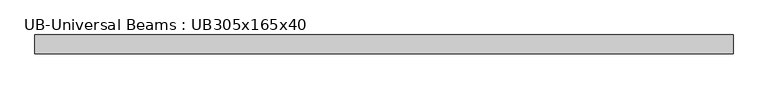
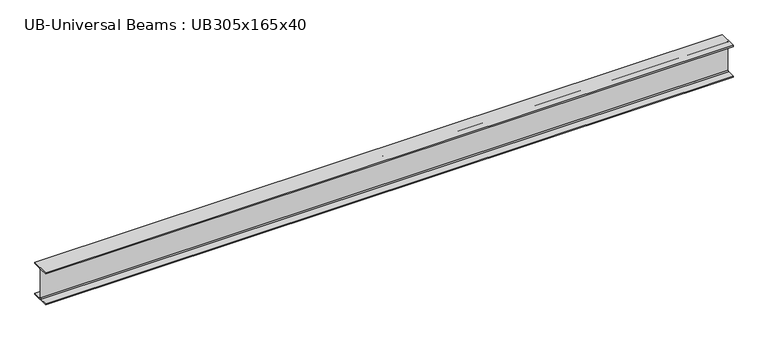
"""IFC4 building model written with IfcOpenShell, lengths in millimetres: beam geometry, UB-Universal Beams : UB305x165x40."""

from ifc_helpers import new_model, si_unit, point, frame, frame_2d, origin, place, context, project, spatial, polyline, circle_curve, trimmed, segment, composite_curve, outline, extrude, source, transform, mapped, element, save


def ub_universal_beams_ub305x165x40_44492b97(model_context):
    return source(origin(), model_context, "Body", "SweptSolid", [
        extrude(outline(composite_curve([segment(polyline([(82.5, -141.5), (82.5, -151.7), (-82.5, -151.7), (-82.5, -141.5), (-11.9, -141.5)]), True, "CONTINUOUS"), segment(trimmed(circle_curve(frame_2d((-11.9, -132.6)), 8.9), [point((-11.9, -141.5))], [point((-3.0, -132.6))], True, "CARTESIAN"), True, "CONTINUOUS"), segment(polyline([(-3.0, -132.6), (-3.0, 132.6)]), True, "CONTINUOUS"), segment(trimmed(circle_curve(frame_2d((-11.9, 132.6)), 8.9), [point((-3.0, 132.6))], [point((-11.9, 141.5))], True, "CARTESIAN"), True, "CONTINUOUS"), segment(polyline([(-11.9, 141.5), (-82.5, 141.5), (-82.5, 151.7), (82.5, 151.7), (82.5, 141.5), (11.9, 141.5)]), True, "CONTINUOUS"), segment(trimmed(circle_curve(frame_2d((11.9, 132.6)), 8.9), [point((11.9, 141.5))], [point((3.0, 132.6))], True, "CARTESIAN"), True, "CONTINUOUS"), segment(polyline([(3.0, 132.6), (3.0, -132.6)]), True, "CONTINUOUS"), segment(trimmed(circle_curve(frame_2d((11.9, -132.6)), 8.9), [point((3.0, -132.6))], [point((11.9, -141.5))], True, "CARTESIAN"), True, "CONTINUOUS"), segment(polyline([(11.9, -141.5), (82.5, -141.5)]), True, "CONTINUOUS")], self_intersect=False)), frame((-3187.65, 0.0, 0.0), z_axis=(1.0, 0.0, 0.0), x_axis=(0.0, 1.0, 0.0)), (0.0, 0.0, 1.0), 6165.8),
    ])


if __name__ == "__main__":
    model = new_model("IFC4")
    model_context = context("Model", 3, world=origin())
    ifc_project = project(units=[si_unit("LENGTHUNIT", "METRE", prefix="MILLI")], contexts=[model_context])
    site = spatial("IfcSite", under=ifc_project)
    building = spatial("IfcBuilding", under=site)
    placement = place(None, origin())
    ub_universal_beams_ub305x165x40_shape = ub_universal_beams_ub305x165x40_44492b97(model_context)
    element("IfcBeam", 1, ObjectType="UB-Universal Beams : UB305x165x40", at=placement, inside=building, context=model_context, shape_type="MappedRepresentation", body=[
        mapped(ub_universal_beams_ub305x165x40_shape, transform((0.0, 0.0, 0.0), x_axis=(1.0, 0.0, 0.0), y_axis=(0.0, 1.0, 0.0), z_axis=(0.0, 0.0, 1.0))),
    ])
    save(model, "model.ifc")

# Revit data of these elements
# Type "UB-Universal Beams : UB305x165x40"
#   Section Name Key = "UB305X165X40"
#   Width = 16.5 cm
#   Web Thickness = 0.6 cm
#   Web Fillet = 0.89 cm
#   Warping Constant = 164000.0 cm⁶
#   Torsional Moment of Inertia = 14.70 cm⁴
#   Section Area = 51.3 cm²
#   Plastic Modulus weak axis = 142.0 cm³
#   Plastic Modulus strong axis = 623.0 cm³
#   Nominal Weight = 40.2999 kgf/m
#   Moment of Inertia weak axis = 764.00 cm⁴
#   Moment of Inertia strong axis = 8503.00 cm⁴
#   Height = 30.34 cm
#   Flange Thickness = 1.02 cm
#   Elastic Modulus weak axis = 92.6 cm³
#   Elastic Modulus strong axis = 560.0 cm³
#   Centroid Vertical = 15.17 cm
#   Centroid Horizontal = 8.25 cm
#   Bolt Spacing = 9.0 cm
#   Length [instance default] = 1500 mm
#   Structural Material [instance default] = Metal - Steel 43-275
#   Type Comments = ""
#   Assembly Code = ""
# Element 1 (IfcBeam, "UB-Universal Beams : UB305x165x40")
#   Materials on its faces: "Metal - Steel 43-275"
# Materials
#   "Metal - Steel 43-275": class "Metal", colour RGB 247 247 247, transparency 0, Cost = 0
